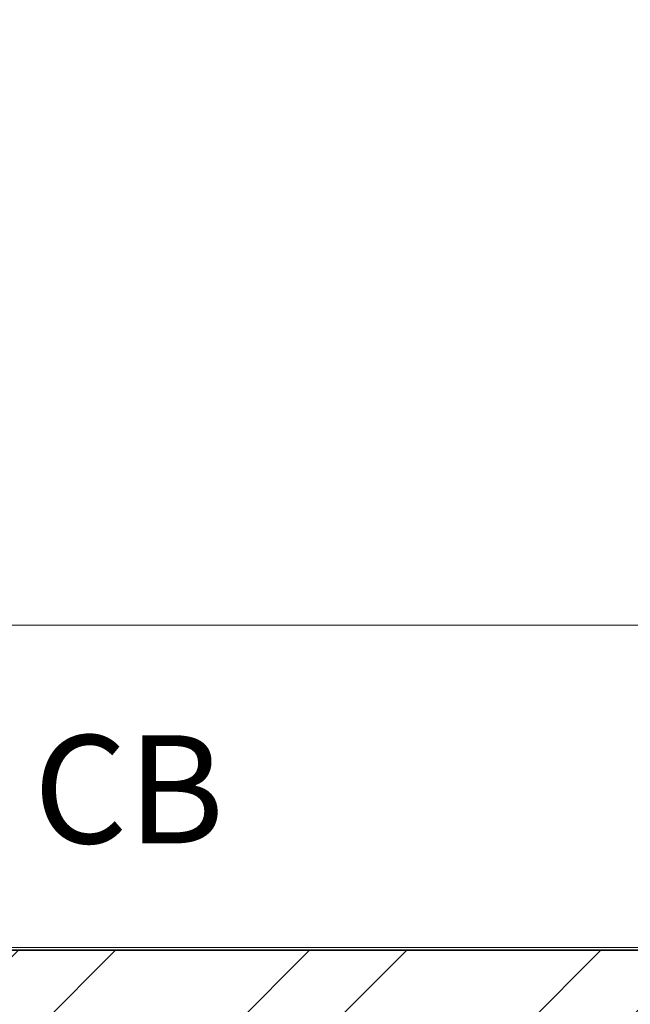
# Model space of a CAD drawing. Units: inches. Extents: x 2168 to 3056, y 1130 to 2629.
# Tile 39 of 42: x 2818 to 2846, y 2263 to 2308. Entities that reach past the tile are written whole.
import ezdxf

# ---------------------------------------------------------------- set-up
doc = ezdxf.new("R2010")
doc.units = ezdxf.units.IN
for name, color, linetype, lineweight in [('A-ANNO-TEXT', 7, 'Continuous', 18), ('A-FLOR-CASE', 71, 'Continuous', 18), ('A-WALL', 7, 'Continuous', 35)]:
    doc.layers.add(name, color=color, linetype=linetype, lineweight=lineweight)
doc.layers.add('A-WALL-PATT', color=143, linetype='Continuous', lineweight=13, true_color=0x7aafdf)
doc.styles.get("Standard").update_dxf_attribs({"font": 'arial.ttf'})

# ---------------------------------------------------------------- blocks, each defined once
blk = doc.blocks.new('CUPBOARD-BEDROOM')
blk.add_lwpolyline([(0, 14.894), (70.359, 14.894), (70.359, 0), (0, 0)], close=True)

msp = doc.modelspace()

# ---------------------------------------------------------------- hatches: boundary and pattern name
at = {"layer": 'A-WALL-PATT'}
h = msp.add_hatch(dxfattribs=at)
h.set_pattern_fill('ANSI32', color=256)
h.paths.add_polyline_path([(2463.796, 2409.389), (2467.387, 2409.389), (2467.387, 2413.889), (2454.768, 2413.889), (2454.768, 2411.639), (2454.768, 2409.389), (2459.296, 2409.389), (2459.296, 2265.389), (2455.644, 2265.389), (2455.644, 2260.889), (2467.349, 2260.889), (2467.349, 2263.139), (2467.349, 2265.389), (2463.796, 2265.389)])
h.paths.add_polyline_path([(2431.596, 2413.889), (2409.647, 2413.889), (2409.647, 2409.389), (2431.596, 2409.389), (2431.596, 2411.639)])
h.paths.add_polyline_path([(2349.647, 2413.889), (2331.796, 2413.889), (2331.796, 2362.671), (2336.296, 2362.671), (2336.296, 2409.389), (2349.647, 2409.389), (2349.647, 2411.639)])
h.paths.add_polyline_path([(2634.149, 2411.639), (2634.149, 2413.889), (2562.293, 2413.889), (2562.293, 2409.389), (2595.796, 2409.389), (2595.796, 2280.309), (2595.826, 2280.309), (2595.826, 2265.389), (2499.91, 2265.389), (2499.91, 2260.889), (2550.796, 2260.889), (2550.796, 2117.308), (2555.296, 2117.308), (2555.296, 2168.08), (2571.93, 2168.08), (2571.93, 2176.889), (2559.796, 2176.889), (2559.796, 2256.389), (2640.796, 2256.389), (2640.796, 2176.889), (2626.428, 2176.889), (2626.428, 2168.08), (2645.296, 2168.08), (2645.296, 2116.637), (2649.796, 2116.637), (2649.796, 2260.889), (2691.251, 2260.889), (2691.251, 2263.139), (2691.251, 2265.389), (2670.655, 2265.389), (2670.655, 2265.365), (2600.296, 2265.365), (2600.296, 2280.258), (2600.296, 2409.389), (2634.149, 2409.389)])
h.paths.add_polyline_path([(2600.296, 2473.889), (2612.84, 2473.889), (2612.84, 2478.389), (2572.636, 2478.389), (2572.636, 2473.889), (2595.796, 2473.889), (2595.796, 2413.889), (2600.296, 2413.889)])
h.paths.add_polyline_path([(2535.796, 2473.889), (2548.636, 2473.889), (2548.636, 2478.389), (2531.396, 2478.389), (2531.396, 2413.889), (2521.6, 2413.889), (2521.6, 2409.389), (2539.239, 2409.389), (2539.239, 2411.639), (2539.239, 2413.889), (2535.796, 2413.889)])
h.paths.add_polyline_path([(2664.796, 2478.389), (2636.84, 2478.389), (2636.84, 2473.889), (2660.296, 2473.889), (2660.296, 2413.889), (2656.165, 2413.889), (2656.165, 2409.389), (2671.684, 2409.389), (2671.684, 2411.639), (2671.684, 2413.889), (2664.796, 2413.889)])
h.paths.add_polyline_path([(2705.942, 2413.889), (2695.684, 2413.889), (2695.684, 2409.389), (2705.942, 2409.389)])
h.paths.add_polyline_path([(2741.35, 2413.889), (2728.733, 2413.889), (2728.733, 2411.639), (2728.733, 2409.389), (2732.296, 2409.389), (2732.296, 2265.389), (2725.733, 2265.389), (2725.733, 2260.889), (2740.917, 2260.889), (2740.917, 2263.139), (2740.917, 2265.389), (2736.796, 2265.389), (2736.796, 2409.389), (2741.35, 2409.389)])
h.paths.add_polyline_path([(2785.655, 2413.889), (2764.546, 2413.889), (2764.486, 2409.389), (2785.655, 2409.389), (2785.655, 2411.639)])
h.paths.add_polyline_path([(2864.296, 2413.889), (2845.655, 2413.889), (2845.655, 2409.389), (2859.796, 2409.389), (2859.796, 2368.425), (2864.296, 2368.425)])
h.paths.add_polyline_path([(2864.296, 2308.425), (2862.046, 2308.425), (2859.796, 2308.425), (2859.796, 2265.389), (2774.483, 2265.389), (2774.483, 2263.139), (2774.483, 2260.889), (2781.796, 2260.889), (2781.796, 2226.654), (2786.296, 2226.654), (2786.296, 2260.889), (2859.796, 2260.889), (2859.796, 2241.352), (2864.296, 2241.352)])
h.paths.add_polyline_path([(2864.296, 2217.352), (2862.046, 2217.352), (2859.796, 2217.352), (2859.796, 2200.889), (2786.296, 2200.889), (2786.296, 2205.931), (2784.046, 2205.931), (2781.796, 2205.931), (2781.796, 2150.974), (2786.296, 2150.974), (2786.296, 2161.889), (2859.796, 2161.889), (2859.796, 2144.419), (2864.296, 2144.419)])
h.paths.add_polyline_path([(2859.796, 2196.389), (2859.796, 2166.389), (2786.296, 2166.389), (2786.296, 2196.389)], flags=16)
h.paths.add_polyline_path([(2864.296, 2108.419), (2862.046, 2108.419), (2859.796, 2108.419), (2859.796, 2080.889), (2786.296, 2080.889), (2786.296, 2111.993), (2781.796, 2111.993), (2781.796, 2080.889), (2649.796, 2080.889), (2649.796, 2086.036), (2647.546, 2086.036), (2645.296, 2086.036), (2645.296, 2071.739), (2649.796, 2071.739), (2649.796, 2076.389), (2781.796, 2076.389), (2781.796, 2041.792), (2786.296, 2041.792), (2786.296, 2076.389), (2859.796, 2076.389), (2859.796, 2058.577), (2864.296, 2058.577)])
h.paths.add_polyline_path([(2864.296, 2022.577), (2859.796, 2022.577), (2859.796, 1992.389), (2786.296, 1992.389), (2786.296, 1999.573), (2781.796, 1999.573), (2781.796, 1848.085), (2784.046, 1848.085), (2786.296, 1848.085), (2786.296, 1851.389), (2859.796, 1851.389), (2859.796, 1838.258), (2864.296, 1838.258)], flags=17)
h.paths.add_polyline_path([(2859.796, 1987.889), (2859.796, 1855.889), (2786.296, 1855.889), (2786.296, 1987.889)], flags=16)
h.paths.add_polyline_path([(2823.046, 1987.889), (2841.421, 1921.889), (2823.046, 1855.889)], flags=0)
h.paths.add_polyline_path([(2864.296, 1814.258), (2859.796, 1814.258), (2859.796, 1791.389), (2786.296, 1791.389), (2786.296, 1825.658), (2784.046, 1825.658), (2781.796, 1825.658), (2781.796, 1791.389), (2720.155, 1791.389), (2720.155, 1791.265), (2649.796, 1791.265), (2649.796, 1806.159), (2649.796, 2038.983), (2647.546, 2038.983), (2645.296, 2038.983), (2645.296, 1783.925), (2649.796, 1783.925), (2649.796, 1786.889), (2781.796, 1786.889), (2781.796, 1746.789), (2786.296, 1746.789), (2786.296, 1786.889), (2859.796, 1786.889), (2859.796, 1770.083), (2864.296, 1770.083)])
h.paths.add_polyline_path([(2864.296, 1734.083), (2862.046, 1734.083), (2859.796, 1734.083), (2859.796, 1705.889), (2786.296, 1705.889), (2786.296, 1714.166), (2781.796, 1714.166), (2781.796, 1660.527), (2786.296, 1660.527), (2786.296, 1666.889), (2859.796, 1666.889), (2859.796, 1648.342), (2864.296, 1648.342)])
h.paths.add_polyline_path([(2786.296, 1701.389), (2859.796, 1701.389), (2859.796, 1671.389), (2786.296, 1671.389)], flags=16)
h.paths.add_polyline_path([(2649.796, 1756.576), (2647.546, 1756.576), (2645.296, 1756.576), (2645.296, 1606.889), (2555.296, 1606.889), (2555.296, 1749.513), (2553.046, 1749.513), (2550.796, 1749.513), (2550.796, 1606.889), (2503.006, 1606.889), (2503.006, 1604.639), (2503.006, 1602.389), (2595.796, 1602.389), (2595.849, 1602.389), (2595.849, 1587.495), (2595.796, 1458.389), (2561.502, 1458.389), (2561.502, 1456.139), (2561.502, 1453.889), (2595.796, 1453.889), (2595.796, 1381.889), (2573.438, 1381.889), (2573.438, 1377.389), (2613.01, 1377.389), (2613.01, 1379.639), (2613.01, 1381.889), (2600.296, 1381.889), (2600.296, 1453.889), (2634.327, 1453.889), (2634.327, 1458.389), (2600.296, 1458.389), (2600.296, 1602.389), (2670.655, 1602.389), (2694.095, 1602.389), (2694.095, 1606.889), (2649.796, 1606.889)])
h.paths.add_polyline_path([(2736.796, 1602.389), (2741.562, 1602.389), (2741.562, 1606.889), (2726.203, 1606.889), (2726.203, 1604.639), (2726.203, 1602.389), (2732.296, 1602.389), (2732.296, 1458.389), (2727.899, 1458.389), (2727.899, 1453.889), (2740.821, 1453.889), (2740.821, 1456.139), (2740.821, 1458.389), (2736.796, 1458.389)])
h.paths.add_polyline_path([(2859.796, 1606.889), (2786.296, 1606.889), (2786.296, 1637.334), (2784.046, 1637.334), (2781.796, 1637.334), (2781.796, 1606.889), (2775.612, 1606.889), (2775.612, 1602.389), (2859.796, 1602.389)])
h.paths.add_polyline_path([(2864.296, 1624.342), (2862.046, 1624.342), (2859.796, 1624.342), (2859.796, 1570.39), (2864.296, 1570.39)])
h.paths.add_polyline_path([(2864.296, 1510.39), (2862.046, 1510.39), (2859.796, 1510.39), (2859.796, 1458.389), (2846.735, 1458.389), (2846.735, 1456.139), (2846.735, 1453.889), (2864.296, 1453.889)])
h.paths.add_polyline_path([(2786.735, 1458.389), (2765.444, 1458.389), (2765.444, 1453.889), (2786.735, 1453.889)])
h.paths.add_polyline_path([(2706.004, 1458.389), (2695.36, 1458.389), (2695.36, 1453.889), (2706.004, 1453.889), (2706.004, 1456.139)])
h.paths.add_polyline_path([(2671.36, 1456.139), (2671.36, 1458.389), (2655.986, 1458.389), (2655.986, 1456.139), (2655.986, 1453.889), (2660.296, 1453.889), (2660.296, 1381.889), (2637.01, 1381.889), (2637.01, 1377.389), (2664.796, 1377.389), (2664.796, 1453.889), (2671.36, 1453.889)], flags=17)
h.paths.add_polyline_path([(2539.829, 1458.389), (2520.237, 1458.389), (2520.237, 1453.889), (2531.296, 1453.889), (2531.296, 1377.389), (2546.449, 1377.389), (2546.449, 1379.639), (2546.449, 1381.889), (2535.796, 1381.889), (2535.796, 1453.889), (2539.829, 1453.889)], flags=17)
h.paths.add_polyline_path([(2496.237, 1458.389), (2489.13, 1458.389), (2489.13, 1453.889), (2496.237, 1453.889), (2496.237, 1456.139)])
h.paths.add_polyline_path([(2467.433, 1456.139), (2467.433, 1458.389), (2463.796, 1458.389), (2463.796, 1602.389), (2468.242, 1602.389), (2468.242, 1605.7), (2468.242, 1606.889), (2454.602, 1606.889), (2454.602, 1602.389), (2459.296, 1602.389), (2459.296, 1458.389), (2454.24, 1458.389), (2454.24, 1453.889), (2467.433, 1453.889)])
h.paths.add_polyline_path([(2431.601, 1456.139), (2431.601, 1458.389), (2411.386, 1458.389), (2411.386, 1453.889), (2431.601, 1453.889)])
h.paths.add_polyline_path([(2351.386, 1458.389), (2336.296, 1458.389), (2336.296, 1490.693), (2334.046, 1490.693), (2331.796, 1490.693), (2331.796, 1453.889), (2351.386, 1453.889), (2351.386, 1456.139)])
h.paths.add_polyline_path([(2336.296, 1629.705), (2331.796, 1629.705), (2331.796, 1552.317), (2336.296, 1552.317), (2336.296, 1602.389), (2406.655, 1602.389), (2423.472, 1602.389), (2423.472, 1606.889), (2418.796, 1606.889), (2418.796, 1643.678), (2416.546, 1643.678), (2414.296, 1643.678), (2414.296, 1606.889), (2336.296, 1606.889)])
h.paths.add_polyline_path([(2418.796, 1714.384), (2414.296, 1714.384), (2414.296, 1705.889), (2336.296, 1705.889), (2336.296, 1731.324), (2334.046, 1731.324), (2331.796, 1731.324), (2331.796, 1653.705), (2334.046, 1653.705), (2336.296, 1653.705), (2336.296, 1666.889), (2414.296, 1666.889), (2414.296, 1663.589), (2418.796, 1663.589)])
h.paths.add_polyline_path([(2336.296, 1701.389), (2414.296, 1701.389), (2414.296, 1671.389), (2336.296, 1671.389)], flags=16)
h.paths.add_polyline_path([(2555.296, 2040.059), (2550.796, 2040.059), (2550.796, 1791.389), (2550.561, 1791.205), (2480.202, 1791.205), (2418.796, 1791.389), (2418.796, 1825.448), (2416.546, 1825.448), (2414.296, 1825.448), (2414.296, 1791.389), (2336.296, 1791.389), (2336.296, 1806.409), (2331.796, 1806.409), (2331.796, 1767.324), (2336.296, 1767.324), (2336.296, 1786.889), (2414.296, 1786.889), (2414.296, 1745.457), (2418.796, 1745.457), (2418.796, 1786.889), (2550.796, 1786.889), (2550.796, 1783.011), (2555.296, 1783.011)])
h.paths.add_polyline_path([(2418.796, 1923.389), (2423.207, 1923.389), (2423.207, 1925.639), (2423.207, 1927.889), (2418.796, 1927.889), (2418.796, 2000.048), (2414.296, 2000.048), (2414.296, 1992.389), (2336.296, 1992.389), (2336.296, 1987.889), (2414.296, 1987.889), (2414.296, 1855.889), (2336.296, 1855.889), (2336.296, 1851.389), (2414.296, 1851.389), (2414.296, 1846.759), (2418.796, 1846.759)], flags=17)
h.paths.add_polyline_path([(2336.296, 2019.294), (2334.046, 2019.294), (2331.796, 2019.294), (2331.796, 1830.409), (2336.296, 1830.409)], flags=17)
h.paths.add_polyline_path([(2550.796, 1927.889), (2453.541, 1927.889), (2453.541, 1925.639), (2453.541, 1923.389), (2550.796, 1923.389)], flags=17)
h.paths.add_polyline_path([(2744.987, 1927.889), (2649.796, 1927.889), (2649.796, 1923.389), (2744.987, 1923.389), (2744.987, 1925.639)], flags=17)
h.paths.add_polyline_path([(2555.296, 2086.458), (2553.046, 2086.458), (2550.796, 2086.458), (2550.796, 2080.889), (2418.796, 2080.889), (2336.296, 2080.889), (2336.296, 2115.399), (2334.046, 2115.399), (2331.796, 2115.399), (2331.796, 2055.294), (2336.296, 2055.294), (2336.296, 2076.389), (2550.796, 2076.389), (2550.796, 2071.538), (2555.296, 2071.538)])
h.paths.add_polyline_path([(2418.796, 2121.389), (2414.296, 2121.389), (2414.296, 2080.889), (2418.796, 2080.889)])
h.paths.add_polyline_path([(2418.796, 2076.389), (2414.296, 2076.389), (2414.296, 2035.123), (2418.796, 2035.123)])
h.paths.add_polyline_path([(2422.868, 2263.139), (2422.868, 2265.389), (2406.655, 2265.389), (2406.655, 2265.359), (2336.296, 2265.359), (2336.296, 2280.252), (2336.296, 2302.671), (2334.046, 2302.671), (2331.796, 2302.671), (2331.796, 2246.853), (2336.296, 2246.853), (2336.296, 2260.889), (2414.296, 2260.889), (2414.296, 2223.996), (2418.796, 2223.996), (2418.796, 2260.889), (2422.868, 2260.889)])
h.paths.add_polyline_path([(2418.796, 2204.783), (2416.546, 2204.783), (2414.296, 2204.783), (2414.296, 2200.889), (2336.296, 2200.889), (2336.296, 2220.853), (2331.796, 2220.853), (2331.796, 2151.399), (2336.296, 2151.399), (2336.296, 2161.889), (2414.296, 2161.889), (2414.296, 2153.726), (2418.796, 2153.726)])
h.paths.add_polyline_path([(2414.296, 2196.389), (2414.296, 2166.389), (2336.296, 2166.389), (2336.296, 2196.389)], flags=16)
h.paths.add_polyline_path([(2375.296, 2181.389), (2336.296, 2166.389), (2336.296, 2196.389)], flags=0)
h.paths.add_polyline_path([(2809.595, 2172.34), (2838.804, 2172.34), (2838.804, 2190.997), (2809.595, 2190.997)], flags=8)
h.paths.add_polyline_path([(2849.75, 1919.585), (2849.75, 1952.672), (2831.093, 1952.672), (2831.093, 1919.585)], flags=8)
h.paths.add_polyline_path([(2808.875, 1901.967), (2808.875, 1937.85), (2790.149, 1937.85), (2790.149, 1901.967)], flags=8)
h.paths.add_polyline_path([(2806.285, 1671.896), (2835.493, 1671.896), (2835.493, 1690.553), (2806.285, 1690.553)], flags=8)
h.paths.add_polyline_path([(2353.186, 1676.549), (2382.395, 1676.549), (2382.395, 1695.207), (2353.186, 1695.207)], flags=8)
h.paths.add_polyline_path([(2360.083, 1832.308), (2389.241, 1832.308), (2389.241, 1850.966), (2360.083, 1850.966)], flags=25)
h.paths.add_polyline_path([(2354.822, 2167.823), (2384.031, 2167.823), (2384.031, 2186.481), (2354.822, 2186.481)], flags=8)

# ---------------------------------------------------------------- linework, layer by layer
at = {"layer": 'A-WALL'}
msp.add_line((2772.841, 2265.389), (2859.796, 2265.389), dxfattribs=at)

# ---------------------------------------------------------------- block references
at = {"layer": 'A-FLOR-CASE'}
msp.add_blockref('CUPBOARD-BEDROOM', (2789.057, 2265.523), dxfattribs=at)

# ---------------------------------------------------------------- texts
at = {"layer": 'A-ANNO-TEXT', "insert": (2818.364, 2275.334), "char_height": 5, "attachment_point": 1}
msp.add_mtext_dynamic_manual_height_columns('CB', width=82.57932, gutter_width=12.5, heights=[0], dxfattribs=at)

doc.saveas('drawing.dxf')
